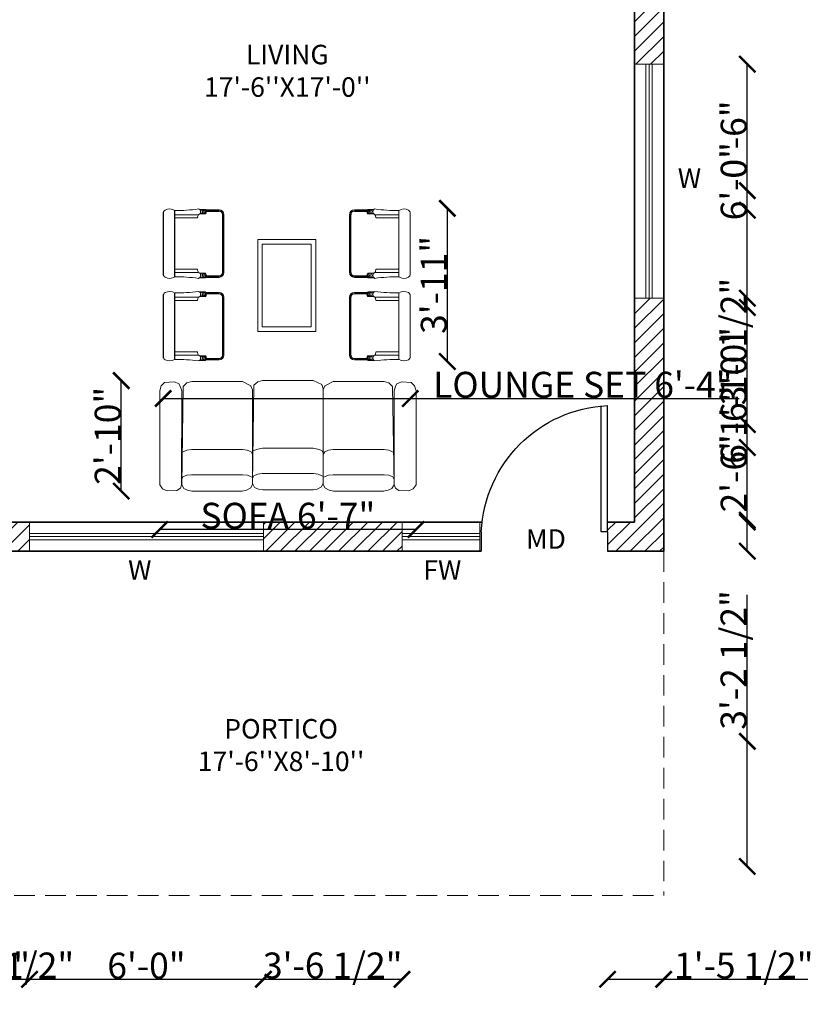
# Model space of a CAD drawing. Units: inches. Extents: x 2094 to 2639, y 1426 to 1997.
# Tile 4 of 8: x 2339 to 2582, y 1426 to 1730. Entities that reach past the tile are written whole.
import ezdxf

# ---------------------------------------------------------------- set-up
doc = ezdxf.new("R2010")
doc.units = ezdxf.units.IN
doc.linetypes.add('HIDDEN', pattern=[9.525, 6.35, -3.175])
for name, color, linetype, lineweight in [('A-ANNO-DIMS', 2, 'Continuous', 18), ('A-ANNO-TEXT', 7, 'Continuous', 18), ('A-AREA-IDEN', 7, 'Continuous', 25), ('A-FLOR-HIDN', 7, 'HIDDEN', 18), ('A-FURN', 8, 'Continuous', 18), ('A-WALL-PATT', 8, 'Continuous', 13), ('Doors', 34, 'Continuous', 25), ('Walls', 7, 'Continuous', 35), ('Windows', 150, 'Continuous', 18)]:
    doc.layers.add(name, color=color, linetype=linetype, lineweight=lineweight)
doc.styles.get("Standard").update_dxf_attribs({"font": 'arial.ttf'})
doc.dimstyles.get("Standard").update_dxf_attribs({"dimtxt": 8, "dimasz": 5, "dimexe": 0.18, "dimexo": 0.0625, "dimgap": 0.09, "dimtad": 1, "dimdec": 1, "dimzin": 0, "dimdsep": 46, "dimlunit": 4, "dimtxsty": 'Standard', "dimblk": 'ARCHTICK', "dimcen": 0.09, "dimse1": 1, "dimse2": 1, "dimadec": 0, "dimazin": 0, "dimtfac": 1, "dimtdec": 1, "dimtofl": 0, "dimtmove": 0, "dimatfit": 3, "dimfxl": 1, "dimtolj": 1, "dimtzin": 0, "dimarcsym": 0})

# ---------------------------------------------------------------- blocks, each defined once
blk = doc.blocks.new('a12')
for p, q in [((1587.145, -521.893), (1587.145, -521.226)), ((1587.148, -521.908), (1587.148, -521.211)), ((1587.271, -521.927), (1587.271, -521.192)), ((1587.273, -521.926), (1587.273, -521.194)), ((1587.273, -521.24), (1587.535, -521.24)), ((1587.546, -521.182), (1587.611, -521.182)), ((1587.549, -521.232), (1587.614, -521.232)), ((1587.616, -521.187), (1587.763, -521.187)), ((1587.622, -521.198), (1587.763, -521.198)), ((1587.624, -521.203), (1587.763, -521.203)), ((1587.8, -521.879), (1587.8, -521.24)), ((1587.805, -521.879), (1587.805, -521.24)), ((1587.816, -521.879), (1587.816, -521.24)), ((1589.204, -521.879), (1589.204, -521.24)), ((1589.215, -521.879), (1589.215, -521.24)), ((1589.22, -521.879), (1589.22, -521.24)), ((1589.404, -521.187), (1589.258, -521.187)), ((1589.398, -521.198), (1589.258, -521.198)), ((1589.397, -521.203), (1589.258, -521.203)), ((1589.471, -521.232), (1589.406, -521.232)), ((1589.475, -521.182), (1589.41, -521.182)), ((1589.748, -521.24), (1589.486, -521.24)), ((1589.748, -521.926), (1589.748, -521.194)), ((1589.75, -521.927), (1589.75, -521.192)), ((1589.873, -521.908), (1589.873, -521.211)), ((1589.876, -521.893), (1589.876, -521.226)), ((1587.273, -521.276), (1587.524, -521.276)), ((1589.748, -521.276), (1589.497, -521.276)), ((1588.19, -521.515), (1588.19, -522.531)), ((1588.831, -521.515), (1588.19, -521.515)), ((1588.78, -521.566), (1588.24, -521.566)), ((1588.24, -521.566), (1588.24, -522.48)), ((1588.78, -522.48), (1588.78, -521.566)), ((1588.831, -522.531), (1588.831, -521.515)), ((1587.273, -521.843), (1587.524, -521.843)), ((1587.273, -521.879), (1587.535, -521.879)), ((1587.549, -521.887), (1587.614, -521.887)), ((1589.471, -521.887), (1589.406, -521.887)), ((1589.748, -521.879), (1589.486, -521.879)), ((1589.748, -521.843), (1589.497, -521.843)), ((1587.546, -521.938), (1587.611, -521.938)), ((1587.616, -521.933), (1587.763, -521.933)), ((1587.622, -521.922), (1587.763, -521.922)), ((1587.624, -521.917), (1587.763, -521.917)), ((1589.397, -521.917), (1589.258, -521.917)), ((1589.398, -521.922), (1589.258, -521.922)), ((1589.404, -521.933), (1589.258, -521.933)), ((1589.475, -521.938), (1589.41, -521.938)), ((1587.271, -522.104), (1587.271, -522.839)), ((1587.273, -522.105), (1587.273, -522.837)), ((1587.546, -522.093), (1587.611, -522.093)), ((1587.616, -522.099), (1587.763, -522.099)), ((1587.622, -522.109), (1587.763, -522.109)), ((1589.404, -522.099), (1589.258, -522.099)), ((1589.398, -522.109), (1589.258, -522.109)), ((1589.475, -522.093), (1589.41, -522.093)), ((1589.748, -522.105), (1589.748, -522.837)), ((1589.75, -522.104), (1589.75, -522.839)), ((1587.145, -522.138), (1587.145, -522.805)), ((1587.148, -522.123), (1587.148, -522.82)), ((1587.273, -522.152), (1587.535, -522.152)), ((1587.273, -522.188), (1587.524, -522.188)), ((1587.549, -522.144), (1587.614, -522.144)), ((1587.624, -522.115), (1587.763, -522.115)), ((1587.8, -522.152), (1587.8, -522.791)), ((1587.805, -522.152), (1587.805, -522.791)), ((1587.816, -522.152), (1587.816, -522.791)), ((1589.204, -522.152), (1589.204, -522.791)), ((1589.215, -522.152), (1589.215, -522.791)), ((1589.22, -522.152), (1589.22, -522.791)), ((1589.397, -522.115), (1589.258, -522.115)), ((1589.471, -522.144), (1589.406, -522.144)), ((1589.748, -522.152), (1589.486, -522.152)), ((1589.748, -522.188), (1589.497, -522.188)), ((1589.873, -522.123), (1589.873, -522.82)), ((1589.876, -522.138), (1589.876, -522.805)), ((1588.19, -522.531), (1588.831, -522.531)), ((1588.24, -522.48), (1588.78, -522.48)), ((1587.273, -522.755), (1587.524, -522.755)), ((1589.748, -522.755), (1589.497, -522.755)), ((1587.273, -522.791), (1587.535, -522.791)), ((1587.546, -522.85), (1587.611, -522.85)), ((1587.549, -522.799), (1587.614, -522.799)), ((1587.616, -522.844), (1587.763, -522.844)), ((1587.622, -522.834), (1587.763, -522.834)), ((1587.624, -522.828), (1587.763, -522.828)), ((1589.397, -522.828), (1589.258, -522.828)), ((1589.398, -522.834), (1589.258, -522.834)), ((1589.404, -522.844), (1589.258, -522.844)), ((1589.471, -522.799), (1589.406, -522.799)), ((1589.475, -522.85), (1589.41, -522.85)), ((1589.748, -522.791), (1589.486, -522.791))]:
    blk.add_line(p, q)
for centre, radius, start, end in [((1587.188, -521.226), 0.0426, 120.0997, 180), ((1587.216, -521.275), 0.0991, 54.9995, 120.0997), ((1587.292, -519.499), 1.695, 269.366, 278.2567), ((1587.604, -521.281), 0.0806, 149.3647, 176.6066), ((1587.526, -521.208), 0.0332, 285.4466, 74.5534), ((1587.53, -521.208), 0.0332, 314.2524, 53.6748), ((1587.547, -521.208), 0.0332, 314.2524, 53.6748), ((1587.563, -521.208), 0.0332, 314.2524, 53.6748), ((1587.576, -521.208), 0.0332, 314.2524, 53.6748), ((1587.585, -521.208), 0.0332, 314.2524, 53.6748), ((1587.589, -521.208), 0.0332, 314.2524, 53.6748), ((1587.591, -521.208), 0.0332, 314.2524, 53.6748), ((1587.763, -521.24), 0.0533, 0, 90), ((1587.763, -521.24), 0.0426, 0, 90), ((1587.763, -521.24), 0.0373, 0, 90), ((1589.258, -521.24), 0.0533, 90, 180), ((1589.258, -521.24), 0.0426, 90, 180), ((1589.258, -521.24), 0.0373, 90, 180), ((1589.43, -521.208), 0.0332, 126.3252, 225.7476), ((1589.432, -521.208), 0.0332, 126.3252, 225.7476), ((1589.435, -521.208), 0.0332, 126.3252, 225.7476), ((1589.445, -521.208), 0.0332, 126.3252, 225.7476), ((1589.458, -521.208), 0.0332, 126.3252, 225.7476), ((1589.473, -521.208), 0.0332, 126.3252, 225.7476), ((1589.491, -521.208), 0.0332, 126.3252, 225.7476), ((1589.494, -521.208), 0.0332, 105.4466, 254.5534), ((1589.729, -519.499), 1.695, 261.7433, 270.634), ((1589.416, -521.281), 0.0806, 3.3934, 30.6353), ((1589.805, -521.275), 0.0991, 59.9003, 125.0005), ((1589.833, -521.226), 0.0426, 0, 59.9003), ((1587.188, -521.893), 0.0426, 180, 239.9003), ((1587.604, -521.838), 0.0806, 183.3934, 210.6353), ((1587.526, -521.911), 0.0332, 285.4466, 74.5534), ((1587.53, -521.911), 0.0332, 306.3252, 45.7476), ((1587.547, -521.911), 0.0332, 306.3252, 45.7476), ((1587.563, -521.911), 0.0332, 306.3252, 45.7476), ((1587.576, -521.911), 0.0332, 306.3252, 45.7476), ((1587.585, -521.911), 0.0332, 306.3252, 45.7476), ((1587.589, -521.911), 0.0332, 306.3252, 45.7476), ((1587.591, -521.911), 0.0332, 306.3252, 45.7476), ((1587.763, -521.879), 0.0373, 270, 0), ((1587.763, -521.879), 0.0533, 270, 0), ((1587.763, -521.879), 0.0533, 270, 0), ((1587.763, -521.879), 0.0426, 270, 0), ((1589.258, -521.879), 0.0533, 180, 270), ((1589.258, -521.879), 0.0533, 180, 270), ((1589.258, -521.879), 0.0426, 180, 270), ((1589.258, -521.879), 0.0373, 180, 270), ((1589.43, -521.911), 0.0332, 134.2524, 233.6748), ((1589.432, -521.911), 0.0332, 134.2524, 233.6748), ((1589.435, -521.911), 0.0332, 134.2524, 233.6748), ((1589.445, -521.911), 0.0332, 134.2524, 233.6748), ((1589.458, -521.911), 0.0332, 134.2524, 233.6748), ((1589.473, -521.911), 0.0332, 134.2524, 233.6748), ((1589.491, -521.911), 0.0332, 134.2524, 233.6748), ((1589.494, -521.911), 0.0332, 105.4466, 254.5534), ((1589.416, -521.838), 0.0806, 329.3647, 356.6066), ((1589.833, -521.893), 0.0426, 300.0997, 0), ((1587.216, -521.845), 0.0991, 239.9003, 305.0005), ((1587.292, -523.621), 1.695, 81.7433, 90.634), ((1589.729, -523.621), 1.695, 89.366, 98.2567), ((1589.805, -521.845), 0.0991, 234.9995, 300.0997), ((1587.188, -522.138), 0.0426, 120.0997, 180), ((1587.216, -522.187), 0.0991, 54.9995, 120.0997), ((1587.292, -520.41), 1.695, 269.366, 278.2567), ((1587.526, -522.12), 0.0332, 285.4466, 74.5534), ((1587.53, -522.12), 0.0332, 314.2524, 53.6748), ((1587.547, -522.12), 0.0332, 314.2524, 53.6748), ((1587.563, -522.12), 0.0332, 314.2524, 53.6748), ((1587.576, -522.12), 0.0332, 314.2524, 53.6748), ((1587.585, -522.12), 0.0332, 314.2524, 53.6748), ((1587.589, -522.12), 0.0332, 314.2524, 53.6748), ((1587.591, -522.12), 0.0332, 314.2524, 53.6748), ((1587.763, -522.152), 0.0533, 0, 90), ((1587.763, -522.152), 0.0533, 0, 90), ((1587.763, -522.152), 0.0426, 0, 90), ((1589.258, -522.152), 0.0533, 90, 180), ((1589.258, -522.152), 0.0533, 90, 180), ((1589.258, -522.152), 0.0426, 90, 180), ((1589.43, -522.12), 0.0332, 126.3252, 225.7476), ((1589.432, -522.12), 0.0332, 126.3252, 225.7476), ((1589.435, -522.12), 0.0332, 126.3252, 225.7476), ((1589.445, -522.12), 0.0332, 126.3252, 225.7476), ((1589.458, -522.12), 0.0332, 126.3252, 225.7476), ((1589.473, -522.12), 0.0332, 126.3252, 225.7476), ((1589.491, -522.12), 0.0332, 126.3252, 225.7476), ((1589.494, -522.12), 0.0332, 105.4466, 254.5534), ((1589.729, -520.41), 1.695, 261.7433, 270.634), ((1589.805, -522.187), 0.0991, 59.9003, 125.0005), ((1589.833, -522.138), 0.0426, 0, 59.9003), ((1587.604, -522.193), 0.0806, 149.3647, 176.6066), ((1587.763, -522.152), 0.0373, 0, 90), ((1589.258, -522.152), 0.0373, 90, 180), ((1589.416, -522.193), 0.0806, 3.3934, 30.6353), ((1587.604, -522.75), 0.0806, 183.3934, 210.6353), ((1589.416, -522.75), 0.0806, 329.3647, 356.6066), ((1587.188, -522.805), 0.0426, 180, 239.9003), ((1587.216, -522.756), 0.0991, 239.9003, 305.0005), ((1587.292, -524.533), 1.695, 81.7433, 90.634), ((1587.526, -522.823), 0.0332, 285.4466, 74.5534), ((1587.53, -522.823), 0.0332, 306.3252, 45.7476), ((1587.547, -522.823), 0.0332, 306.3252, 45.7476), ((1587.563, -522.823), 0.0332, 306.3252, 45.7476), ((1587.576, -522.823), 0.0332, 306.3252, 45.7476), ((1587.585, -522.823), 0.0332, 306.3252, 45.7476), ((1587.589, -522.823), 0.0332, 306.3252, 45.7476), ((1587.591, -522.823), 0.0332, 306.3252, 45.7476), ((1587.763, -522.791), 0.0373, 270, 0), ((1587.763, -522.791), 0.0533, 270, 0), ((1587.763, -522.791), 0.0426, 270, 0), ((1589.258, -522.791), 0.0533, 180, 270), ((1589.258, -522.791), 0.0426, 180, 270), ((1589.258, -522.791), 0.0373, 180, 270), ((1589.43, -522.823), 0.0332, 134.2524, 233.6748), ((1589.432, -522.823), 0.0332, 134.2524, 233.6748), ((1589.435, -522.823), 0.0332, 134.2524, 233.6748), ((1589.445, -522.823), 0.0332, 134.2524, 233.6748), ((1589.458, -522.823), 0.0332, 134.2524, 233.6748), ((1589.473, -522.823), 0.0332, 134.2524, 233.6748), ((1589.491, -522.823), 0.0332, 134.2524, 233.6748), ((1589.494, -522.823), 0.0332, 105.4466, 254.5534), ((1589.729, -524.533), 1.695, 89.366, 98.2567), ((1589.805, -522.756), 0.0991, 234.9995, 300.0997), ((1589.833, -522.805), 0.0426, 300.0997, 0)]:
    blk.add_arc(centre, radius, start, end)
blk = doc.blocks.new('12PCOU17')
at = {"color": 0, "linetype": 'ByBlock'}
for points in [[(-34.71, 34.72), (-33.66, 34.31), (-3.27, 34.3), (-1.81, 34.76), (-1.05, 35.2), (-0.38, 36.65), (-0.61, 39.84), (-1.73, 40.94), (-3.27, 41.4), (-33.66, 41.4), (-34.95, 40.5), (-35.65, 39.02), (-35.49, 35.83), (-34.71, 34.72)], [(-1.89, 11.91), (-1.66, 11.91), (-0.35, 14.68), (-0.35, 31.05), (-0.74, 32.58), (-1.89, 33.83), (-33.63, 34.3), (-34.84, 33.63), (-35.43, 32.38), (-35.68, 31), (-35.68, 14.74), (-35.43, 13.36), (-34.66, 11.99), (-33.44, 11.43), (-3, 11.44), (-1.66, 11.91)], [(-31.25, 11.43), (-31.06, 11.84), (-30.6, 13.09), (-30.4, 14.62), (-30.4, 31.12), (-30.6, 32.65), (-31.06, 33.9), (-31.81, 34.3)], [(-23.84, 11.43), (-22.99, 11.9), (-22.46, 13.15), (-22.23, 14.67), (-22.23, 31.07), (-22.46, 32.59), (-22.99, 33.84), (-23.12, 34.3)], [(-1.54, -10.96), (-1.31, -10.96), (0, -8.19), (0, 8.19), (-0.39, 9.71), (-1.54, 10.96), (-33.28, 11.44), (-34.5, 10.77), (-35.08, 9.51), (-35.33, 8.14), (-35.33, -8.13), (-35.08, -9.51), (-34.31, -10.87), (-33.1, -11.44), (-2.65, -11.43), (-1.31, -10.96)], [(-30.9, -11.44), (-30.72, -11.02), (-30.25, -9.77), (-30.05, -8.25), (-30.05, 8.26), (-30.25, 9.78), (-30.72, 11.03), (-31.47, 11.44)], [(-23.49, -11.44), (-22.64, -10.96), (-22.11, -9.72), (-21.88, -8.19), (-21.88, 8.2), (-22.11, 9.73), (-22.64, 10.97), (-22.77, 11.44)], [(-1.89, -11.91), (-1.66, -11.91), (-0.35, -14.68), (-0.35, -31.05), (-0.74, -32.58), (-1.89, -33.83), (-33.63, -34.3), (-34.84, -33.63), (-35.43, -32.38), (-35.68, -31), (-35.68, -14.74), (-35.43, -13.36), (-34.66, -11.99), (-33.44, -11.43), (-3, -11.44), (-1.66, -11.91)], [(-31.25, -11.43), (-31.06, -11.84), (-30.6, -13.09), (-30.4, -14.62), (-30.4, -31.12), (-30.6, -32.65), (-31.06, -33.9), (-31.81, -34.3)], [(-23.84, -11.43), (-22.99, -11.9), (-22.46, -13.15), (-22.23, -14.67), (-22.23, -31.07), (-22.46, -32.59), (-22.99, -33.84), (-23.12, -34.3)], [(-34.71, -34.72), (-33.66, -34.31), (-3.27, -34.3), (-1.81, -34.76), (-1.05, -35.2), (-0.38, -36.65), (-0.61, -39.84), (-1.73, -40.94), (-3.27, -41.4), (-33.66, -41.4), (-34.95, -40.5), (-35.65, -39.02), (-35.49, -35.83), (-34.71, -34.72)]]:
    blk.add_lwpolyline(points, dxfattribs=at)
blk = doc.blocks.new('AP0B05')
for p, q in [((35, 100), (35, 880)), ((75, 100), (75, 878.9)), ((35, 100), (35, -20)), ((815, 100), (815, -20))]:
    blk.add_line(p, q)
blk.add_lwpolyline([(35, 100), (75, 100)])
blk.add_arc((-2.4, 62.6), 818.3, 2.62122, 87.37878)
blk = doc.blocks.new('WIN-24IN')
for p, q in [((24, 5.5), (0, 5.5)), ((24, 4.5), (0, 4.5)), ((24, 3.5), (0, 3.5))]:
    blk.add_line(p, q)
blk.add_lwpolyline([(24, 9), (0, 9), (0, 0), (24, 0)], close=True)
blk = doc.blocks.new('_ArchTick')
at = {"color": 0, "linetype": 'ByBlock', "const_width": 0.15}
blk.add_lwpolyline([(-0.5, -0.5), (0.5, 0.5)], dxfattribs=at)
blk = doc.blocks.new('*D47')
at = {"layer": 'A-ANNO-DIMS', "color": 0, "lineweight": -2, "transparency": 16777216}
blk.add_line((2460.84, 1572.59), (2381.91, 1572.59), dxfattribs=at)
at = {"layer": 'Defpoints', "color": 0, "transparency": 16777216}
for p in [(2381.91, 1584.43), (2460.84, 1584.43), (2381.91, 1572.59)]:
    blk.add_point(p, dxfattribs=at)
at = {"layer": 'A-ANNO-DIMS', "color": 0, "lineweight": -2, "transparency": 16777216, "xscale": 5, "yscale": 5, "zscale": 5, "rotation": 180}
blk.add_blockref('_ArchTick', (2381.91, 1572.59), dxfattribs=at)
at = {"layer": 'A-ANNO-DIMS', "color": 0, "lineweight": -2, "transparency": 16777216, "xscale": 5, "yscale": 5, "zscale": 5}
blk.add_blockref('_ArchTick', (2460.84, 1572.59), dxfattribs=at)
at = {"layer": 'A-ANNO-DIMS', "color": 0, "transparency": 16777216, "insert": (2421.37, 1576.82), "char_height": 8, "attachment_point": 5}
blk.add_mtext('\\A1;SOFA 6\'-7"', dxfattribs=at)
blk = doc.blocks.new('*D48')
at = {"layer": 'A-ANNO-DIMS', "color": 0, "lineweight": -2, "transparency": 16777216}
blk.add_line((2370.07, 1584.43), (2370.07, 1618.44), dxfattribs=at)
at = {"layer": 'Defpoints', "color": 0, "transparency": 16777216}
for p in [(2370.07, 1618.44), (2381.91, 1618.44), (2381.91, 1584.43)]:
    blk.add_point(p, dxfattribs=at)
at = {"layer": 'A-ANNO-DIMS', "color": 0, "lineweight": -2, "transparency": 16777216, "xscale": 5, "yscale": 5, "zscale": 5}
for p, rotation in [((2370.07, 1618.44), 90), ((2370.07, 1584.43), 270)]:
    blk.add_blockref('_ArchTick', p, dxfattribs=dict(at, rotation=rotation))
at = {"layer": 'A-ANNO-DIMS', "color": 0, "transparency": 16777216, "insert": (2365.9, 1601.43), "char_height": 8, "attachment_point": 5, "rotation": 90}
blk.add_mtext('\\A1;2\'-10"', dxfattribs=at)
blk = doc.blocks.new('*D51')
at = {"layer": 'A-ANNO-DIMS', "color": 0, "lineweight": -2, "transparency": 16777216}
for p, q in [((2382.97, 1612.9), (2459.05, 1612.9)), ((2459.05, 1612.9), (2560.29, 1612.9))]:
    blk.add_line(p, q, dxfattribs=at)
at = {"layer": 'Defpoints', "color": 0, "transparency": 16777216}
for p in [(2382.97, 1624.32), (2459.05, 1624.32), (2459.05, 1612.9)]:
    blk.add_point(p, dxfattribs=at)
at = {"layer": 'A-ANNO-DIMS', "color": 0, "lineweight": -2, "transparency": 16777216, "xscale": 5, "yscale": 5, "zscale": 5, "rotation": 180}
blk.add_blockref('_ArchTick', (2382.97, 1612.9), dxfattribs=at)
at = {"layer": 'A-ANNO-DIMS', "color": 0, "lineweight": -2, "transparency": 16777216, "xscale": 5, "yscale": 5, "zscale": 5}
blk.add_blockref('_ArchTick', (2459.05, 1612.9), dxfattribs=at)
at = {"layer": 'A-ANNO-DIMS', "color": 0, "transparency": 16777216, "insert": (2512.17, 1617.13), "char_height": 8, "attachment_point": 5}
blk.add_mtext('\\A1;LOUNGE SET 6\'-4"', dxfattribs=at)
blk = doc.blocks.new('*D52')
at = {"layer": 'A-ANNO-DIMS', "color": 0, "lineweight": -2, "transparency": 16777216}
blk.add_line((2470.47, 1624.32), (2470.47, 1671.44), dxfattribs=at)
at = {"layer": 'Defpoints', "color": 0, "transparency": 16777216}
for p in [(2459.05, 1671.44), (2470.47, 1671.44), (2459.05, 1624.32)]:
    blk.add_point(p, dxfattribs=at)
at = {"layer": 'A-ANNO-DIMS', "color": 0, "lineweight": -2, "transparency": 16777216, "xscale": 5, "yscale": 5, "zscale": 5}
for p, rotation in [((2470.47, 1671.44), 90), ((2470.47, 1624.32), 270)]:
    blk.add_blockref('_ArchTick', p, dxfattribs=dict(at, rotation=rotation))
at = {"layer": 'A-ANNO-DIMS', "color": 0, "transparency": 16777216, "insert": (2466.29, 1647.88), "char_height": 8, "attachment_point": 5, "rotation": 90}
blk.add_mtext('\\A1;3\'-11"', dxfattribs=at)
blk = doc.blocks.new('*D59')
at = {"layer": 'A-ANNO-DIMS', "color": 0, "lineweight": -2, "transparency": 16777216}
blk.add_line((2562.81, 1565.9), (2562.81, 1643.81), dxfattribs=at)
at = {"layer": 'Defpoints', "color": 0, "transparency": 16777216}
for p in [(2537.06, 1643.81), (2562.81, 1643.81), (2537.06, 1565.9)]:
    blk.add_point(p, dxfattribs=at)
at = {"layer": 'A-ANNO-DIMS', "color": 0, "lineweight": -2, "transparency": 16777216, "xscale": 5, "yscale": 5, "zscale": 5}
for p, rotation in [((2562.81, 1643.81), 90), ((2562.81, 1565.9), 270)]:
    blk.add_blockref('_ArchTick', p, dxfattribs=dict(at, rotation=rotation))
at = {"layer": 'A-ANNO-DIMS', "color": 0, "transparency": 16777216, "insert": (2558.63, 1604.86), "char_height": 8, "attachment_point": 5, "rotation": 90}
blk.add_mtext('\\A1;6\'-6"', dxfattribs=at)
blk = doc.blocks.new('*D60')
at = {"layer": 'A-ANNO-DIMS', "color": 0, "lineweight": -2, "transparency": 16777216}
blk.add_line((2562.81, 1643.81), (2562.81, 1715.81), dxfattribs=at)
at = {"layer": 'Defpoints', "color": 0, "transparency": 16777216}
for p in [(2537.06, 1715.81), (2562.81, 1715.81), (2537.06, 1643.81)]:
    blk.add_point(p, dxfattribs=at)
at = {"layer": 'A-ANNO-DIMS', "color": 0, "lineweight": -2, "transparency": 16777216, "xscale": 5, "yscale": 5, "zscale": 5}
for p, rotation in [((2562.81, 1715.81), 90), ((2562.81, 1643.81), 270)]:
    blk.add_blockref('_ArchTick', p, dxfattribs=dict(at, rotation=rotation))
at = {"layer": 'A-ANNO-DIMS', "color": 0, "transparency": 16777216, "insert": (2558.63, 1679.81), "char_height": 8, "attachment_point": 5, "rotation": 90}
blk.add_mtext('\\A1;6\'-0"', dxfattribs=at)
blk = doc.blocks.new('*D61')
at = {"layer": 'A-ANNO-DIMS', "color": 0, "lineweight": -2, "transparency": 16777216}
blk.add_line((2318.06, 1434.15), (2341.83, 1434.15), dxfattribs=at)
at = {"layer": 'Defpoints', "color": 0, "transparency": 16777216}
for p in [(2318.06, 1565.9), (2341.83, 1565.9), (2341.83, 1434.15)]:
    blk.add_point(p, dxfattribs=at)
at = {"layer": 'A-ANNO-DIMS', "color": 0, "lineweight": -2, "transparency": 16777216, "xscale": 5, "yscale": 5, "zscale": 5, "rotation": 180}
blk.add_blockref('_ArchTick', (2318.06, 1434.15), dxfattribs=at)
at = {"layer": 'A-ANNO-DIMS', "color": 0, "lineweight": -2, "transparency": 16777216, "xscale": 5, "yscale": 5, "zscale": 5}
blk.add_blockref('_ArchTick', (2341.83, 1434.15), dxfattribs=at)
at = {"layer": 'A-ANNO-DIMS', "color": 0, "transparency": 16777216, "insert": (2329.94, 1438.32), "char_height": 8, "attachment_point": 5}
blk.add_mtext('\\A1;2\'-0"', dxfattribs=at)
blk = doc.blocks.new('*D62')
at = {"layer": 'A-ANNO-DIMS', "color": 0, "lineweight": -2, "transparency": 16777216}
blk.add_line((2341.83, 1434.15), (2413.83, 1434.15), dxfattribs=at)
at = {"layer": 'Defpoints', "color": 0, "transparency": 16777216}
for p in [(2341.83, 1565.9), (2413.83, 1565.9), (2413.83, 1434.15)]:
    blk.add_point(p, dxfattribs=at)
at = {"layer": 'A-ANNO-DIMS', "color": 0, "lineweight": -2, "transparency": 16777216, "xscale": 5, "yscale": 5, "zscale": 5, "rotation": 180}
blk.add_blockref('_ArchTick', (2341.83, 1434.15), dxfattribs=at)
at = {"layer": 'A-ANNO-DIMS', "color": 0, "lineweight": -2, "transparency": 16777216, "xscale": 5, "yscale": 5, "zscale": 5}
blk.add_blockref('_ArchTick', (2413.83, 1434.15), dxfattribs=at)
at = {"layer": 'A-ANNO-DIMS', "color": 0, "transparency": 16777216, "insert": (2377.83, 1438.32), "char_height": 8, "attachment_point": 5}
blk.add_mtext('\\A1;6\'-0"', dxfattribs=at)
blk = doc.blocks.new('*D63')
at = {"layer": 'A-ANNO-DIMS', "color": 0, "lineweight": -2, "transparency": 16777216}
blk.add_line((2413.83, 1434.15), (2456.51, 1434.15), dxfattribs=at)
at = {"layer": 'Defpoints', "color": 0, "transparency": 16777216}
for p in [(2413.83, 1565.9), (2456.51, 1565.9), (2456.51, 1434.15)]:
    blk.add_point(p, dxfattribs=at)
at = {"layer": 'A-ANNO-DIMS', "color": 0, "lineweight": -2, "transparency": 16777216, "xscale": 5, "yscale": 5, "zscale": 5, "rotation": 180}
blk.add_blockref('_ArchTick', (2413.83, 1434.15), dxfattribs=at)
at = {"layer": 'A-ANNO-DIMS', "color": 0, "lineweight": -2, "transparency": 16777216, "xscale": 5, "yscale": 5, "zscale": 5}
blk.add_blockref('_ArchTick', (2456.51, 1434.15), dxfattribs=at)
at = {"layer": 'A-ANNO-DIMS', "color": 0, "transparency": 16777216, "insert": (2435.17, 1438.38), "char_height": 8, "attachment_point": 5}
blk.add_mtext('\\A1;3\'-6 1/2"', dxfattribs=at)
blk = doc.blocks.new('*D64')
at = {"layer": 'A-ANNO-DIMS', "color": 0, "lineweight": -2, "transparency": 16777216}
for p, q in [((2519.78, 1434.15), (2537.06, 1434.15)), ((2537.06, 1434.15), (2581.39, 1434.15))]:
    blk.add_line(p, q, dxfattribs=at)
at = {"layer": 'Defpoints', "color": 0, "transparency": 16777216}
for p in [(2519.78, 1565.9), (2537.06, 1565.9), (2537.06, 1434.15)]:
    blk.add_point(p, dxfattribs=at)
at = {"layer": 'A-ANNO-DIMS', "color": 0, "lineweight": -2, "transparency": 16777216, "xscale": 5, "yscale": 5, "zscale": 5, "rotation": 180}
blk.add_blockref('_ArchTick', (2519.78, 1434.15), dxfattribs=at)
at = {"layer": 'A-ANNO-DIMS', "color": 0, "lineweight": -2, "transparency": 16777216, "xscale": 5, "yscale": 5, "zscale": 5}
blk.add_blockref('_ArchTick', (2537.06, 1434.15), dxfattribs=at)
at = {"layer": 'A-ANNO-DIMS', "color": 0, "transparency": 16777216, "insert": (2561.72, 1438.37), "char_height": 8, "attachment_point": 5}
blk.add_mtext('\\A1;1\'-5 1/2"', dxfattribs=at)
blk = doc.blocks.new('*D65')
at = {"layer": 'A-ANNO-DIMS', "color": 0, "lineweight": -2, "transparency": 16777216}
blk.add_line((2562.81, 1604.9), (2562.81, 1640.9), dxfattribs=at)
at = {"layer": 'Defpoints', "color": 0, "transparency": 16777216}
for p in [(2318.06, 1640.9), (2562.81, 1640.9), (2318.06, 1604.9)]:
    blk.add_point(p, dxfattribs=at)
at = {"layer": 'A-ANNO-DIMS', "color": 0, "lineweight": -2, "transparency": 16777216, "xscale": 5, "yscale": 5, "zscale": 5}
for p, rotation in [((2562.81, 1640.9), 90), ((2562.81, 1604.9), 270)]:
    blk.add_blockref('_ArchTick', p, dxfattribs=dict(at, rotation=rotation))
at = {"layer": 'A-ANNO-DIMS', "color": 0, "transparency": 16777216, "insert": (2558.63, 1622.9), "char_height": 8, "attachment_point": 5, "rotation": 90}
blk.add_mtext('\\A1;3\'-0"', dxfattribs=at)
blk = doc.blocks.new('*D67')
at = {"layer": 'A-ANNO-DIMS', "color": 0, "lineweight": -2, "transparency": 16777216}
for p, q in [((2562.81, 1676.9), (2562.81, 1703.34)), ((2562.81, 1670.9), (2562.81, 1676.9))]:
    blk.add_line(p, q, dxfattribs=at)
at = {"layer": 'Defpoints', "color": 0, "transparency": 16777216}
for p in [(2309.06, 1676.9), (2562.81, 1676.9), (2309.06, 1670.9)]:
    blk.add_point(p, dxfattribs=at)
at = {"layer": 'A-ANNO-DIMS', "color": 0, "lineweight": -2, "transparency": 16777216, "xscale": 5, "yscale": 5, "zscale": 5}
for p, rotation in [((2562.81, 1676.9), 90), ((2562.81, 1670.9), 270)]:
    blk.add_blockref('_ArchTick', p, dxfattribs=dict(at, rotation=rotation))
at = {"layer": 'A-ANNO-DIMS', "color": 0, "transparency": 16777216, "insert": (2558.63, 1692.62), "char_height": 8, "attachment_point": 5, "rotation": 90}
blk.add_mtext('\\A1;0\'-6"', dxfattribs=at)
blk = doc.blocks.new('*D69')
at = {"layer": 'A-ANNO-DIMS', "color": 0, "lineweight": -2, "transparency": 16777216}
blk.add_line((2562.81, 1574.9), (2562.81, 1604.9), dxfattribs=at)
at = {"layer": 'Defpoints', "color": 0, "transparency": 16777216}
for p in [(2318.06, 1604.9), (2562.81, 1604.9), (2318.06, 1574.9)]:
    blk.add_point(p, dxfattribs=at)
at = {"layer": 'A-ANNO-DIMS', "color": 0, "lineweight": -2, "transparency": 16777216, "xscale": 5, "yscale": 5, "zscale": 5}
for p, rotation in [((2562.81, 1604.9), 90), ((2562.81, 1574.9), 270)]:
    blk.add_blockref('_ArchTick', p, dxfattribs=dict(at, rotation=rotation))
at = {"layer": 'A-ANNO-DIMS', "color": 0, "transparency": 16777216, "insert": (2558.63, 1589.9), "char_height": 8, "attachment_point": 5, "rotation": 90}
blk.add_mtext('\\A1;2\'-6"', dxfattribs=at)
blk = doc.blocks.new('*D71')
at = {"layer": 'A-ANNO-DIMS', "color": 0, "lineweight": -2, "transparency": 16777216}
for p, q in [((2300.69, 1434.15), (2309.06, 1434.15)), ((2309.06, 1434.15), (2354.14, 1434.15))]:
    blk.add_line(p, q, dxfattribs=at)
at = {"layer": 'Defpoints', "color": 0, "transparency": 16777216}
for p in [(2300.69, 1576.98), (2309.06, 1574.9), (2309.06, 1434.15)]:
    blk.add_point(p, dxfattribs=at)
at = {"layer": 'A-ANNO-DIMS', "color": 0, "lineweight": -2, "transparency": 16777216, "xscale": 5, "yscale": 5, "zscale": 5, "rotation": 180}
blk.add_blockref('_ArchTick', (2300.69, 1434.15), dxfattribs=at)
at = {"layer": 'A-ANNO-DIMS', "color": 0, "lineweight": -2, "transparency": 16777216, "xscale": 5, "yscale": 5, "zscale": 5}
blk.add_blockref('_ArchTick', (2309.06, 1434.15), dxfattribs=at)
at = {"layer": 'A-ANNO-DIMS', "color": 0, "transparency": 16777216, "insert": (2334.1, 1438.37), "char_height": 8, "attachment_point": 5}
blk.add_mtext('\\A1;0\'-8 1/2"', dxfattribs=at)
blk = doc.blocks.new('*D74')
at = {"layer": 'A-ANNO-DIMS', "color": 0, "lineweight": -2, "transparency": 16777216}
for p, q in [((2562.81, 1597.81), (2562.81, 1648.35)), ((2562.81, 1575.5), (2562.81, 1597.81))]:
    blk.add_line(p, q, dxfattribs=at)
at = {"layer": 'Defpoints', "color": 0, "transparency": 16777216}
for p in [(2261.92, 1597.81), (2562.81, 1597.81), (2261.92, 1575.5)]:
    blk.add_point(p, dxfattribs=at)
at = {"layer": 'A-ANNO-DIMS', "color": 0, "lineweight": -2, "transparency": 16777216, "xscale": 5, "yscale": 5, "zscale": 5}
for p, rotation in [((2562.81, 1597.81), 90), ((2562.81, 1575.5), 270)]:
    blk.add_blockref('_ArchTick', p, dxfattribs=dict(at, rotation=rotation))
at = {"layer": 'A-ANNO-DIMS', "color": 0, "transparency": 16777216, "insert": (2558.58, 1625.58), "char_height": 8, "attachment_point": 5, "rotation": 90}
blk.add_mtext('\\A1;1\'-10 1/2"', dxfattribs=at)
blk = doc.blocks.new('*D77')
at = {"layer": 'A-ANNO-DIMS', "color": 0, "lineweight": -2, "transparency": 16777216}
for p, q in [((2308.06, 1954.65), (2318.06, 1954.65)), ((2318.06, 1954.65), (2350.72, 1954.65))]:
    blk.add_line(p, q, dxfattribs=at)
at = {"layer": 'Defpoints', "color": 0, "transparency": 16777216}
for p in [(2318.06, 1954.65), (2308.06, 1468.9), (2318.06, 1468.9)]:
    blk.add_point(p, dxfattribs=at)
at = {"layer": 'A-ANNO-DIMS', "color": 0, "lineweight": -2, "transparency": 16777216, "xscale": 5, "yscale": 5, "zscale": 5, "rotation": 180}
blk.add_blockref('_ArchTick', (2308.06, 1954.65), dxfattribs=at)
at = {"layer": 'A-ANNO-DIMS', "color": 0, "lineweight": -2, "transparency": 16777216, "xscale": 5, "yscale": 5, "zscale": 5}
blk.add_blockref('_ArchTick', (2318.06, 1954.65), dxfattribs=at)
at = {"layer": 'A-ANNO-DIMS', "color": 0, "transparency": 16777216, "insert": (2336.89, 1958.82), "char_height": 8, "attachment_point": 5}
blk.add_mtext('\\A1;0\'-10"', dxfattribs=at)
blk = doc.blocks.new('*D78')
at = {"layer": 'A-ANNO-DIMS', "color": 0, "lineweight": -2, "transparency": 16777216}
for p, q in [((2562.81, 1507.4), (2562.81, 1552.48)), ((2562.81, 1468.9), (2562.81, 1507.4))]:
    blk.add_line(p, q, dxfattribs=at)
at = {"layer": 'Defpoints', "color": 0, "transparency": 16777216}
for p in [(2318.06, 1507.4), (2562.81, 1507.4), (2318.06, 1468.9)]:
    blk.add_point(p, dxfattribs=at)
at = {"layer": 'A-ANNO-DIMS', "color": 0, "lineweight": -2, "transparency": 16777216, "xscale": 5, "yscale": 5, "zscale": 5}
for p, rotation in [((2562.81, 1507.4), 90), ((2562.81, 1468.9), 270)]:
    blk.add_blockref('_ArchTick', p, dxfattribs=dict(at, rotation=rotation))
at = {"layer": 'A-ANNO-DIMS', "color": 0, "transparency": 16777216, "insert": (2558.58, 1532.44), "char_height": 8, "attachment_point": 5, "rotation": 90}
blk.add_mtext('\\A1;3\'-2 1/2"', dxfattribs=at)

msp = doc.modelspace()

# ---------------------------------------------------------------- hatches: boundary and pattern name
at = {"layer": 'A-WALL-PATT', "transparency": 33554585}
h = msp.add_hatch(dxfattribs=at)
h.set_pattern_fill('ANSI31', color=256)
h.paths.add_polyline_path([(2189.06, 1727.9), (2230.3, 1727.9, -0.022928), (2230.09, 1730.2), (2230.09, 1733.9), (2189.06, 1733.9), (2189.06, 1742.37), (2180.06, 1742.37), (2180.06, 1714.4), (2189.06, 1714.4)])
h.paths.add_polyline_path([(2456.51, 1574.9), (2413.83, 1574.9), (2413.83, 1565.9), (2456.51, 1565.9)])
h.paths.add_polyline_path([(2537.06, 1643.81), (2528.06, 1643.81), (2528.06, 1574.9), (2519.78, 1574.9), (2519.78, 1571.88), (2519.78, 1565.9), (2537.06, 1565.9)])
h.paths.add_polyline_path([(2339.06, 1928.9), (2300.94, 1928.9), (2300.94, 1919.9), (2309.06, 1919.9), (2309.06, 1776.3, -0.024186), (2312.62, 1776.64), (2318.06, 1776.64), (2318.06, 1778.9), (2336.06, 1778.9), (2336.06, 1787.9), (2318.06, 1787.9), (2318.06, 1835.9), (2384.06, 1835.9), (2384.06, 1787.9), (2366.06, 1787.9), (2366.06, 1778.9), (2479.64, 1778.9), (2479.64, 1784.88, -0.018603), (2479.89, 1787.9), (2390.06, 1787.9), (2390.06, 1847.57), (2385.61, 1847.57), (2384.06, 1847.57), (2384.06, 1841.9), (2318.06, 1841.9), (2318.06, 1919.9), (2339.06, 1919.9)])
h.paths.add_polyline_path([(2252.94, 1928.9), (2180.06, 1928.9), (2180.06, 1790.37), (2189.06, 1790.37), (2189.06, 1843.77), (2189.06, 1919.9), (2252.94, 1919.9)])
h.paths.add_polyline_path([(2472.33, 1928.9), (2363.06, 1928.9), (2363.06, 1919.9), (2384.06, 1919.9), (2384.06, 1876.38, -0.012802), (2385.61, 1876.49), (2390.06, 1876.49), (2390.06, 1919.9), (2472.33, 1919.9)], flags=17)
h.paths.add_polyline_path([(2537.06, 1928.9), (2520.33, 1928.9), (2520.33, 1919.9), (2528.06, 1919.9), (2528.06, 1905.95), (2528.06, 1787.9), (2518.5, 1787.9), (2518.5, 1784.88), (2518.5, 1778.9), (2528.06, 1778.9), (2528.06, 1715.81), (2537.06, 1715.81)])
h.paths.add_polyline_path([(2379.33, 1857.12), (2393.06, 1857.12), (2393.06, 1866.16), (2379.33, 1866.16)], flags=25)
h.paths.add_polyline_path([(2235.85, 1725.77), (2249.57, 1725.77), (2249.57, 1734.81), (2235.85, 1734.81)], flags=25)
h.paths.add_polyline_path([(2305.79, 1754.6), (2314.84, 1754.6), (2314.84, 1763.6), (2305.79, 1763.6)], flags=9)
h.paths.add_polyline_path([(2493.85, 1778.22), (2502.9, 1778.22), (2502.9, 1787.22), (2493.85, 1787.22)], flags=9)
h.paths.add_polyline_path([(2370.69, 1555.65), (2381.6, 1555.65), (2381.6, 1564.65), (2370.69, 1564.65)], flags=9)
h.paths.add_polyline_path([(2461.57, 1555.65), (2477.6, 1555.65), (2477.6, 1564.65), (2461.57, 1564.65)], flags=9)
h.paths.add_polyline_path([(2493.18, 1565.15), (2509.22, 1565.15), (2509.22, 1574.15), (2493.18, 1574.15)], flags=9)
h.paths.add_polyline_path([(2408.32, 1501.7), (2449.12, 1501.7), (2449.12, 1520.36), (2408.32, 1520.36)], flags=9)
h.paths.add_polyline_path([(2398.49, 1698.6), (2441.61, 1698.6), (2441.61, 1717.26), (2398.49, 1717.26)], flags=9)
h.paths.add_polyline_path([(2248.63, 1683.29), (2287.87, 1683.29), (2287.87, 1701.95), (2248.63, 1701.95)], flags=25)
h.paths.add_polyline_path([(2440.73, 1823.2), (2483.86, 1823.2), (2483.86, 1841.85), (2440.73, 1841.85)], flags=9)
h.paths.add_polyline_path([(2335.3, 1804.5), (2370.65, 1804.5), (2370.65, 1823.15), (2335.3, 1823.15)], flags=25)
h.paths.add_polyline_path([(2335.3, 1893.12), (2370.65, 1893.12), (2370.65, 1911.77), (2335.3, 1911.77)], flags=25)
h.paths.add_polyline_path([(2241.82, 1863.6), (2290.11, 1863.6), (2290.11, 1882.25), (2241.82, 1882.25)], flags=9)
h = msp.add_hatch(dxfattribs=at)
h.set_pattern_fill('ANSI31', color=256)
h.paths.add_polyline_path([(2318.06, 1741.32), (2312.62, 1741.32), (2309.06, 1741.32), (2309.06, 1733.9), (2254.12, 1733.9), (2254.12, 1730.2), (2254.12, 1727.9), (2309.06, 1727.9), (2309.06, 1676.9), (2189.06, 1676.9), (2189.06, 1690.4), (2180.06, 1690.4), (2180.06, 1646.9), (2189.06, 1646.9), (2189.06, 1670.9), (2309.06, 1670.9), (2309.06, 1640.9), (2318.06, 1640.9)])
h.paths.add_polyline_path([(2318.06, 1604.9), (2309.06, 1604.9), (2309.06, 1574.9), (2189.06, 1574.9), (2189.06, 1598.9), (2180.06, 1598.9), (2180.06, 1459.9), (2318.06, 1459.9), (2318.06, 1468.9), (2189.06, 1468.9), (2189.06, 1565.9), (2341.83, 1565.9), (2341.83, 1574.9), (2318.06, 1574.9)])

# ---------------------------------------------------------------- linework, layer by layer
at = {"layer": 'A-FLOR-HIDN'}
for p in [(2537.06, 1565.9), (2318.06, 1459.9)]:
    msp.add_line(p, (2537.06, 1459.9), dxfattribs=at)
at = {"layer": 'Walls'}
for p, q in [((2537.06, 1928.9), (2537.06, 1565.9)), ((2528.06, 1778.9), (2528.06, 1574.9)), ((2318.06, 1574.9), (2481.17, 1574.9)), ((2519.78, 1574.9), (2528.06, 1574.9)), ((2189.06, 1565.9), (2480.92, 1565.9)), ((2519.78, 1565.9), (2537.06, 1565.9))]:
    msp.add_line(p, q, dxfattribs=at)
at = {"layer": 'Windows'}
for p, q in [((2531.56, 1715.81), (2531.56, 1643.81)), ((2532.56, 1715.81), (2532.56, 1643.81)), ((2533.56, 1715.81), (2533.56, 1643.81)), ((2413.83, 1571.4), (2341.83, 1571.4)), ((2413.83, 1570.4), (2341.83, 1570.4)), ((2413.83, 1569.4), (2341.83, 1569.4))]:
    msp.add_line(p, q, dxfattribs=at)
for points in [[(2528.06, 1715.81), (2528.06, 1643.81), (2537.06, 1643.81), (2537.06, 1715.81)], [(2413.83, 1574.9), (2341.83, 1574.9), (2341.83, 1565.9), (2413.83, 1565.9)]]:
    msp.add_lwpolyline(points, close=True, dxfattribs=at)

# ---------------------------------------------------------------- block references
at = {"layer": 'A-FURN', "xscale": 27.86263550351131, "yscale": 27.86263550351131, "zscale": 27.86263550351131}
msp.add_blockref('a12', (-41839.07, 16192.61), dxfattribs=at)
at = {"layer": 'A-FURN', "xscale": 0.9531824723496688, "yscale": 0.9531824723496688, "zscale": 0.9531824723496688, "rotation": 90}
msp.add_blockref('12PCOU17', (2421.37, 1618.44), dxfattribs=at)
at = {"layer": 'Doors', "xscale": -0.0498171271707621, "yscale": 0.0498171271707621, "zscale": 0.0498171271707621}
msp.add_blockref('AP0B05', (2521.52, 1566.89), dxfattribs=at)
at = {"layer": 'Windows'}
msp.add_blockref('WIN-24IN', (2456.51, 1565.9), dxfattribs=at)

# ---------------------------------------------------------------- texts
at = {"layer": 'A-ANNO-TEXT'}
for s, p in [('W', (2541.41, 1677.72)), ('MD', (2494.68, 1566.65)), ('W', (2372.19, 1557.15)), ('FW', (2463.07, 1557.15))]:
    msp.add_text(s, height=6, dxfattribs=at).set_placement(p)
at = {"layer": 'A-AREA-IDEN', "char_height": 6, "attachment_point": 1}
for s, insert in [("\\pxqc;LIVING\\P17'-6''X17'-0''", (2394.64, 1721.79)), ("\\pxqc;PORTICO\\P17'-6''X8'-10''", (2392.73, 1514.25))]:
    msp.add_mtext_dynamic_manual_height_columns(s, width=53.0999, gutter_width=63.55, heights=[0], dxfattribs=dict(at, insert=insert))

# ---------------------------------------------------------------- dimensions: what is measured, and where the dimension line sits
at = {"layer": 'A-ANNO-DIMS'}
for base, p1, p2, picture, middle in [((2318.06, 1954.65), (2308.06, 1468.9), (2318.06, 1468.9), '*D77', (2336.89, 1958.82)), ((2309.06, 1434.15), (2300.69, 1576.98), (2309.06, 1574.9), '*D71', (2334.1, 1438.37)), ((2341.83, 1434.15), (2318.06, 1565.9), (2341.83, 1565.9), '*D61', (2329.94, 1438.32)), ((2413.83, 1434.15), (2341.83, 1565.9), (2413.83, 1565.9), '*D62', (2377.83, 1438.32)), ((2456.51, 1434.15), (2413.83, 1565.9), (2456.51, 1565.9), '*D63', (2435.17, 1438.38)), ((2537.06, 1434.15), (2519.78, 1565.9), (2537.06, 1565.9), '*D64', (2561.72, 1438.37))]:
    dim = msp.add_linear_dim(base=base, p1=p1, p2=p2, dimstyle='Standard', override={"dimdec": 1, "dimlfac": 1, "dimrnd": 0, "dimzin": 1, "dimdsep": 46, "dimlunit": 4, "dimfrac": 2}, dxfattribs=at)
    dim.commit()
    dim.dimension.update_dxf_attribs({"geometry": picture, "text_midpoint": middle})
for base, p1, p2, picture, middle in [((2562.81, 1715.81), (2537.06, 1643.81), (2537.06, 1715.81), '*D60', (2558.63, 1679.81)), ((2562.81, 1676.9), (2309.06, 1670.9), (2309.06, 1676.9), '*D67', (2558.63, 1692.62)), ((2470.47, 1671.44), (2459.05, 1624.32), (2459.05, 1671.44), '*D52', (2466.29, 1647.88)), ((2562.81, 1597.81), (2261.92, 1575.5), (2261.92, 1597.81), '*D74', (2558.58, 1625.58)), ((2562.81, 1643.81), (2537.06, 1565.9), (2537.06, 1643.81), '*D59', (2558.63, 1604.86)), ((2562.81, 1640.9), (2318.06, 1604.9), (2318.06, 1640.9), '*D65', (2558.63, 1622.9)), ((2370.07, 1618.44), (2381.91, 1584.43), (2381.91, 1618.44), '*D48', (2365.9, 1601.43)), ((2562.81, 1604.9), (2318.06, 1574.9), (2318.06, 1604.9), '*D69', (2558.63, 1589.9)), ((2562.81, 1507.4), (2318.06, 1468.9), (2318.06, 1507.4), '*D78', (2558.58, 1532.44))]:
    dim = msp.add_linear_dim(base=base, p1=p1, p2=p2, angle=90, dimstyle='Standard', override={"dimdec": 1, "dimlfac": 1, "dimrnd": 0, "dimzin": 1, "dimdsep": 46, "dimlunit": 4, "dimfrac": 2}, dxfattribs=at)
    dim.commit()
    dim.dimension.update_dxf_attribs({"geometry": picture, "text_midpoint": middle})
dim = msp.add_linear_dim(base=(2459.05, 1612.9), p1=(2382.97, 1624.32), p2=(2459.05, 1624.32), text='LOUNGE SET <>', dimstyle='Standard', override={"dimdec": 1, "dimlfac": 1, "dimrnd": 0, "dimzin": 1, "dimdsep": 46, "dimlunit": 4, "dimfrac": 2}, dxfattribs=at)
dim.commit()
dim.dimension.update_dxf_attribs({"geometry": '*D51', "text_midpoint": (2512.17, 1617.13)})
dim = msp.add_linear_dim(base=(2381.91, 1572.59), p1=(2460.84, 1584.43), p2=(2381.91, 1584.43), angle=180, text='SOFA <>', dimstyle='Standard', override={"dimdec": 1, "dimlfac": 1, "dimrnd": 0, "dimzin": 1, "dimdsep": 46, "dimlunit": 4, "dimfrac": 2}, dxfattribs=at)
dim.commit()
dim.dimension.update_dxf_attribs({"geometry": '*D47', "text_midpoint": (2421.37, 1576.82)})

doc.saveas('drawing.dxf')
